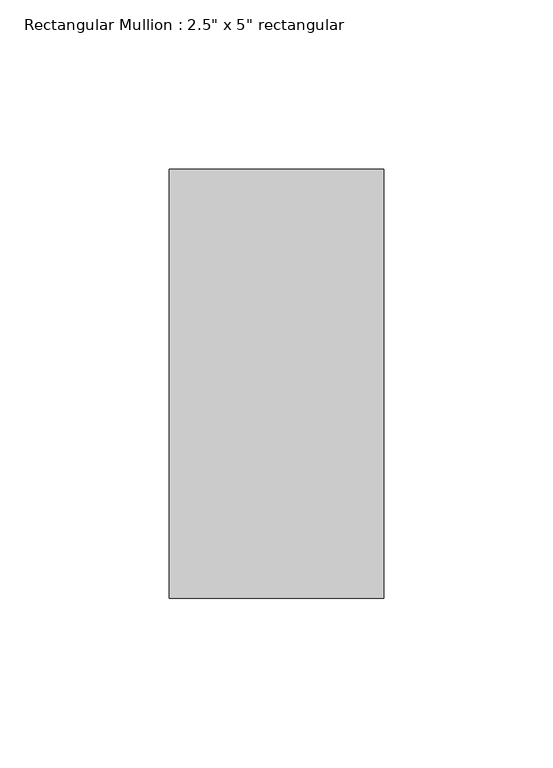
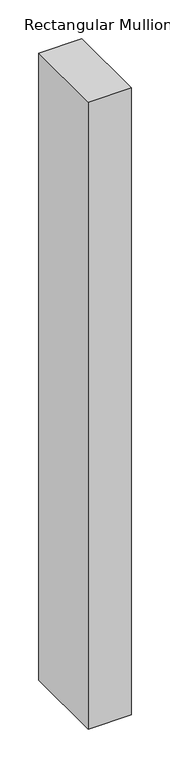
"""IFC4 building model written with IfcOpenShell, lengths in millimetres: member geometry."""

from ifc_helpers import new_model, si_unit, frame, origin, place, context, project, spatial, polyline, outline, extrude, source, transform, mapped, element, save


def member_f5f6c3fe(model_context):
    return source(origin(), model_context, "Body", "SweptSolid", [
        extrude(outline(polyline([(0.0, 63.5), (0.0, -63.5), (-63.5, -63.5), (-63.5, 63.5), (0.0, 63.5)])), frame((0.0, 0.0, -984.25), z_axis=(0.0, 0.0, 1.0), x_axis=(1.0, 0.0, 0.0)), (0.0, 0.0, 1.0), 984.25),
    ])


if __name__ == "__main__":
    model = new_model("IFC4")
    model_context = context("Model", 3, world=origin())
    ifc_project = project(units=[si_unit("LENGTHUNIT", "METRE", prefix="MILLI")], contexts=[model_context])
    site = spatial("IfcSite", under=ifc_project)
    building = spatial("IfcBuilding", under=site)
    placement = place(None, origin())
    member_shape = member_f5f6c3fe(model_context)
    element("IfcMember", 1, ObjectType="Rectangular Mullion : 2.5\" x 5\" rectangular", at=placement, inside=building, context=model_context, shape_type="MappedRepresentation", body=[
        mapped(member_shape, transform((0.0, 0.0, 0.0), x_axis=(1.0, 0.0, 0.0), y_axis=(0.0, 1.0, 0.0), z_axis=(0.0, 0.0, 1.0))),
    ])
    save(model, "model.ifc")

# Revit data of these elements
# Type "Rectangular Mullion : 2.5\" x 5\" rectangular"
#   built-in parameter 1007304 = 0.416667 (stored number, unit not read)
#   built-in parameter 1007301 = 0.104167 (stored number, unit not read)
#   built-in parameter 1007300 = 0.104167 (stored number, unit not read)
# Element 1 (IfcMember, "Rectangular Mullion : 2.5\" x 5\" rectangular")
#   Materials on its faces: "Aluminum"
# Materials
#   "Aluminum": class "Metal", colour RGB 247 247 247, transparency 0, Description = "Aluminum 6061", Cost = 0
